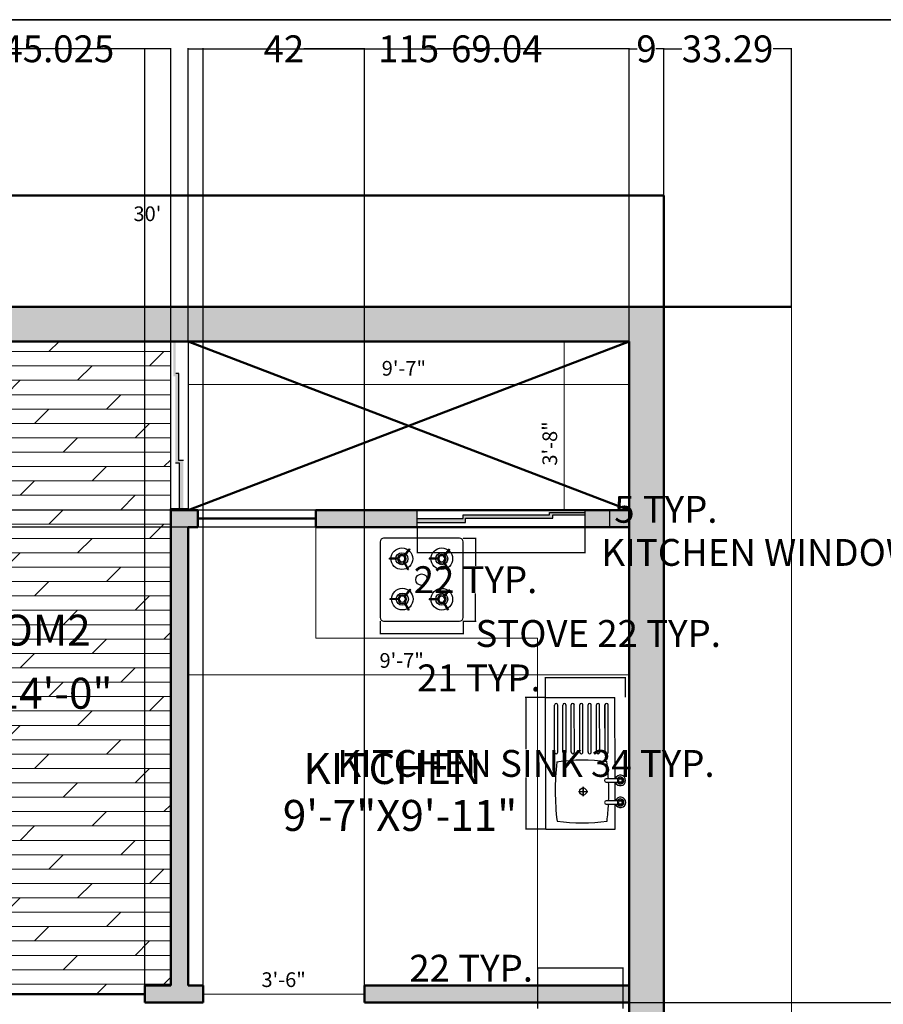
# Model space of a CAD drawing. Units: inches. Extents: x 1381 to 2246, y 1317 to 2168.
# Tile 8 of 15: x 1579 to 1804, y 1911 to 2168. Entities that reach past the tile are written whole.
import ezdxf

# ---------------------------------------------------------------- set-up
doc = ezdxf.new("R2010")
doc.units = ezdxf.units.IN
doc.header["$MEASUREMENT"] = 0
doc.layers.get('0').update_dxf_attribs({"color": 253})
for name, color, linetype, lineweight in [('A-ANNO-DIMS', 2, 'Continuous', 18), ('A-ANNO-TEXT', 7, 'Continuous', 18), ('A-ANNO-TTLB', 7, 'Continuous', 35), ('A-AREA-IDEN', 3, 'Continuous', 25), ('A-FLOR-FIXT', 9, 'Continuous', 18), ('A-FLOR-PATT', 252, 'Continuous', 13), ('A-FURN', 8, 'Continuous', 18), ('A-GLAZ', 4, 'Continuous', 25), ('A-WALL', 7, 'Continuous', 50)]:
    doc.layers.add(name, color=color, linetype=linetype, lineweight=lineweight)
doc.layers.add('furniture', color=250, linetype='Continuous')
doc.styles.get("Standard").update_dxf_attribs({"font": 'arial.ttf'})
doc.dimstyles.get("Standard").update_dxf_attribs({"dimtxt": 7, "dimasz": 0.18, "dimexe": 0.18, "dimexo": 0.0625, "dimgap": 0.09, "dimtad": 0, "dimtih": 1, "dimtoh": 1, "dimdec": 1, "dimzin": 0, "dimdsep": 46, "dimlunit": 3, "dimtxsty": 'Standard', "dimcen": 0.09, "dimadec": 0, "dimazin": 0, "dimtfac": 1, "dimtdec": 1, "dimtofl": 0, "dimtmove": 0, "dimatfit": 3, "dimfxl": 1, "dimtolj": 1, "dimtzin": 0, "dimarcsym": 0})

# ---------------------------------------------------------------- blocks, each defined once
blk = doc.blocks.new('4bstove')
at = {"layer": 'furniture'}
for p, q in [((1452.73, 1446.21), (1452.73, 1448.61)), ((1452.98, 1446.22), (1452.98, 1448.61)), ((1464.44, 1446.34), (1464.44, 1448.73)), ((1464.69, 1446.34), (1464.69, 1448.73)), ((1451.74, 1444.45), (1449.67, 1443.25)), ((1451.87, 1444.23), (1449.79, 1443.04)), ((1453.75, 1444.08), (1455.58, 1442.54)), ((1453.91, 1444.27), (1455.74, 1442.73)), ((1463.45, 1444.58), (1461.38, 1443.38)), ((1463.57, 1444.36), (1461.5, 1443.17)), ((1465.46, 1444.21), (1467.29, 1442.67)), ((1465.62, 1444.4), (1467.45, 1442.86)), ((1452.69, 1434.81), (1452.69, 1437.2)), ((1452.94, 1434.81), (1452.94, 1437.2)), ((1464.44, 1434.81), (1464.44, 1437.2)), ((1464.69, 1434.81), (1464.69, 1437.2)), ((1451.7, 1433.04), (1449.63, 1431.85)), ((1451.82, 1432.83), (1449.75, 1431.63)), ((1453.71, 1432.67), (1455.54, 1431.13)), ((1453.87, 1432.86), (1455.7, 1431.33)), ((1463.45, 1433.04), (1461.38, 1431.85)), ((1463.57, 1432.83), (1461.5, 1431.63)), ((1465.46, 1432.67), (1467.29, 1431.13)), ((1465.62, 1432.86), (1467.45, 1431.33))]:
    blk.add_line(p, q, dxfattribs=at)
for points in [[(1447.5, 1427.38), (1469.5, 1427.38, 0.414214), (1470.5, 1428.38), (1470.5, 1450.38, 0.414214), (1469.5, 1451.38), (1447.5, 1451.38, 0.414214), (1446.5, 1450.38), (1446.5, 1428.38, 0.414214)], [(1453.75, 1444.97, 1), (1452, 1444.97, 1)], [(1465.46, 1445.1, 1), (1463.71, 1445.1, 1)], [(1453.71, 1433.56, 1), (1451.96, 1433.56, 1)], [(1465.46, 1433.56, 1), (1463.71, 1433.56, 1)]]:
    blk.add_lwpolyline(points, format="xyb", close=True, dxfattribs=at)
for points in [[(1454.12, 1444.97, 1), (1451.62, 1444.97, 1), (1454.12, 1444.97, 1)], [(1465.83, 1445.1, 1), (1463.33, 1445.1, 1), (1465.83, 1445.1, 1)], [(1454.08, 1433.56, 1), (1451.58, 1433.56, 1), (1454.08, 1433.56, 1)], [(1465.83, 1433.56, 1), (1463.33, 1433.56, 1), (1465.83, 1433.56, 1)]]:
    blk.add_lwpolyline(points, format="xyb", dxfattribs=at)
for centre, radius in [((1452.87, 1444.97), 3.14), ((1464.58, 1445.1), 3.14), ((1452.87, 1444.97), 1.75), ((1464.58, 1445.1), 1.75), ((1458.5, 1439.38), 1.67), ((1452.83, 1433.56), 3.14), ((1464.58, 1433.56), 3.14), ((1452.83, 1433.56), 1.75), ((1464.58, 1433.56), 1.75)]:
    blk.add_circle(centre, radius, dxfattribs=at)
for centre, start, end in [((1452.87, 1444.97), 88.2645, 92.2039), ((1464.58, 1445.1), 88.2645, 92.2039), ((1452.87, 1444.97), 208.188, 212.1274), ((1452.87, 1444.97), 318.1018, 322.0412), ((1464.58, 1445.1), 208.188, 212.1274), ((1464.58, 1445.1), 318.1018, 322.0412), ((1452.83, 1433.56), 88.2645, 92.2039), ((1464.58, 1433.56), 88.2645, 92.2039)]:
    blk.add_arc(centre, 3.64, start, end, dxfattribs=at)
blk = doc.blocks.new('stove')
at = {"layer": 'furniture', "xscale": 0.9, "yscale": 0.9, "zscale": 0.9, "rotation": 89.99999999999999}
blk.add_blockref('4bstove', (1295.44, -1312.65), dxfattribs=at)
blk = doc.blocks.new('A$C799204C7')
for p, q in [((0, 34.2), (17.99, 34.2)), ((0, 0), (0, 34.2)), ((17.99, 13.08), (17.99, 34.2)), ((2.32, 20.01), (2.32, 32.27)), ((3.13, 20.01), (3.13, 32.27)), ((4.48, 20.01), (4.48, 32.27)), ((5.29, 20.01), (5.29, 32.27)), ((6.64, 20.01), (6.64, 32.27)), ((7.45, 20.01), (7.45, 32.27)), ((8.85, 20.01), (8.85, 32.27)), ((9.66, 20.01), (9.66, 32.27)), ((11.01, 20.01), (11.01, 32.27)), ((11.82, 20.01), (11.82, 32.27)), ((13.22, 20.01), (13.22, 32.27)), ((14.03, 20.01), (14.03, 32.27)), ((15.42, 20.01), (15.42, 32.27)), ((16.24, 20.01), (16.24, 32.27)), ((18.59, 13.08), (15.71, 13.08)), ((9.73, 11), (9.73, 8.54)), ((15.71, 12.17), (18.59, 12.17)), ((17.99, 7.36), (17.99, 12.17)), ((8.52, 9.77), (10.9, 9.77)), ((18.59, 7.36), (15.71, 7.36)), ((15.71, 6.45), (18.59, 6.45)), ((17.99, 0), (17.99, 6.45)), ((0, 0), (17.99, 0))]:
    blk.add_line(p, q)
for centre, radius in [((19.38, 12.62), 0.684), ((19.38, 12.62), 0.456), ((9.7, 9.77), 0.916), ((19.38, 6.91), 0.684), ((19.38, 6.91), 0.456)]:
    blk.add_circle(centre, radius)
for centre, radius, start, end in [((2.72, 32.27), 0.407, 0, 180), ((4.88, 32.27), 0.407, 0, 180), ((7.05, 32.27), 0.407, 0, 180), ((9.25, 32.27), 0.407, 0, 180), ((11.42, 32.27), 0.407, 0, 180), ((13.62, 32.27), 0.407, 0, 180), ((15.83, 32.27), 0.407, 0, 180), ((2.72, 20.01), 0.407, 180, 0), ((4.88, 20.01), 0.407, 180, 0), ((7.05, 20.01), 0.407, 180, 0), ((9.25, 20.01), 0.407, 180, 0), ((11.42, 20.01), 0.407, 180, 0), ((13.62, 20.01), 0.407, 180, 0), ((15.83, 20.01), 0.407, 180, 0), ((67.33, 9.77), 64.88, 173.1952, 186.8048), ((9.53, -30.19), 48.1, 82.3437, 97.8966), ((-48.51, 9.77), 64.88, 2.9208, 6.8048), ((15.71, 12.62), 0.456, 90, 270), ((19.38, 12.62), 1.37, 199.6514, 160.3603), ((19.38, 12.62), 0.911, 210.3431, 149.7554), ((-48.51, 9.77), 64.88, 357.8723, 2.115), ((19.38, 6.91), 1.37, 199.6514, 160.3603), ((19.38, 6.91), 0.911, 210.3431, 149.7554), ((15.71, 6.91), 0.456, 90, 270), ((-48.51, 9.77), 64.88, 353.1952, 357.0665), ((9.53, 49.73), 48.1, 262.1034, 277.6563)]:
    blk.add_arc(centre, radius, start, end)
blk = doc.blocks.new('sink')
at = {"layer": 'furniture'}
for p, q in [((8718164203.894819, -1433730582.369047), (8718164201.504578, -1433730582.369047)), ((8718164202.684322, -1433730581.131674), (8718164202.684322, -1433730583.598095)), ((8718164196.150837, -1433730592.638258), (8718164196.150837, -1433730604.938997)), ((8718164196.967728, -1433730592.638258), (8718164196.967728, -1433730604.938997)), ((8718164198.365185, -1433730592.638258), (8718164198.365185, -1433730604.938997)), ((8718164199.182076, -1433730592.638258), (8718164199.182076, -1433730604.938997)), ((8718164200.579533, -1433730592.638258), (8718164200.579533, -1433730604.938997)), ((8718164201.396423, -1433730592.638258), (8718164201.396423, -1433730604.938997)), ((8718164202.748692, -1433730592.638258), (8718164202.748692, -1433730604.938997)), ((8718164203.565582, -1433730592.638258), (8718164203.565582, -1433730604.938997)), ((8718164204.963041, -1433730592.638258), (8718164204.963041, -1433730604.938997)), ((8718164205.779934, -1433730592.638258), (8718164205.779934, -1433730604.938997)), ((8718164207.1322, -1433730592.638258), (8718164207.1322, -1433730604.938997)), ((8718164207.949093, -1433730592.638258), (8718164207.949093, -1433730604.938997)), ((8718164209.301359, -1433730592.638258), (8718164209.301359, -1433730604.938997)), ((8718164210.118252, -1433730592.638258), (8718164210.118252, -1433730604.938997))]:
    blk.add_line(p, q, dxfattribs=at)
for centre, radius in [((8718164192.998869, -1433730579.495552), 0.685789), ((8718164192.998869, -1433730579.495552), 0.457192), ((8718164202.715019, -1433730582.369047), 0.919003), ((8718164192.998869, -1433730585.228166), 0.68579), ((8718164192.998869, -1433730585.228166), 0.68579), ((8718164192.998869, -1433730585.228166), 0.457192)]:
    blk.add_circle(centre, radius, dxfattribs=at)
for centre, radius, start, end in [((8718164196.559284, -1433730592.638258), 0.41045, 354.3355999, 185.6644001), ((8718164198.77363, -1433730592.638258), 0.41045, 354.3355999, 185.6644001), ((8718164200.98798, -1433730592.638258), 0.41045, 354.3355999, 185.6644001), ((8718164203.157139, -1433730592.638258), 0.41045, 354.3355999, 185.6644001), ((8718164205.371487, -1433730592.638258), 0.41045, 354.3355999, 185.6644001), ((8718164207.540646, -1433730592.640262), 0.41045, 354.3355999, 185.6644001), ((8718164209.709805, -1433730592.640262), 0.41045, 354.3355999, 185.6644001), ((8718164196.559284, -1433730604.938997), 0.408445, 180, 0), ((8718164198.77363, -1433730604.938997), 0.408445, 180, 0), ((8718164200.98798, -1433730604.938997), 0.408445, 180, 0), ((8718164203.157139, -1433730604.938997), 0.408445, 180, 0), ((8718164205.371487, -1433730604.938997), 0.408445, 180, 0), ((8718164207.540646, -1433730604.938997), 0.408445, 180, 0), ((8718164209.709805, -1433730604.938997), 0.408445, 180, 0)]:
    blk.add_arc(centre, radius, start, end, dxfattribs=at)
at = {"layer": 'furniture', "xscale": 1.0032, "yscale": 1.0032, "zscale": 1.0032, "rotation": 180}
blk.add_blockref('A$C799204C7', (8718164212.441259, -1433730572.566334), dxfattribs=at)
blk = doc.blocks.new('washbasin')
at = {"layer": 'furniture'}
blk.add_blockref('sink', (-8718164214.119328, 1433730589.721069), dxfattribs=at)
blk = doc.blocks.new('WIN-KITCHEN')
for p, q in [((0, 0), (0, 4.5)), ((0, 4.5), (43.68, 4.5)), ((43.68, 4.5), (43.68, 0)), ((43.68, 0), (0, 0))]:
    blk.add_line(p, q)
blk = doc.blocks.new('*D30')
at = {"layer": 'A-ANNO-DIMS', "color": 0, "lineweight": -2, "transparency": 16777216}
for p, q in [((1713.7, 1920.4), (1713.52, 1920.4)), ((1713.7, 1909.87), (1713.7, 1920.58)), ((1735.75, 1920.4), (1713.88, 1920.4)), ((1735.93, 1909.87), (1735.93, 1920.58))]:
    blk.add_line(p, q, dxfattribs=at)
at = {"layer": 'A-ANNO-DIMS', "color": 0, "transparency": 16777216}
for points in [[(1713.88, 1920.43), (1713.88, 1920.37), (1713.7, 1920.4)], [(1735.75, 1920.43), (1735.75, 1920.37), (1735.93, 1920.4)]]:
    blk.add_solid(points, dxfattribs=at)
at = {"layer": 'Defpoints', "color": 0, "transparency": 16777216}
for p in [(1713.7, 1920.4), (1713.7, 1909.81), (1735.93, 1909.81)]:
    blk.add_point(p, dxfattribs=at)
at = {"layer": 'A-ANNO-DIMS', "color": 0, "transparency": 16777216, "insert": (1696.34, 1920.4), "char_height": 7, "attachment_point": 5}
blk.add_mtext('\\A1;22 TYP.', dxfattribs=at)
blk = doc.blocks.new('*D31')
at = {"layer": 'A-ANNO-DIMS', "color": 0, "lineweight": -2, "transparency": 16777216}
for p, q in [((1672.63, 2010.89), (1672.63, 2007.53)), ((1694.23, 2010.89), (1694.23, 2007.53)), ((1672.81, 2007.71), (1694.05, 2007.71)), ((1694.23, 2007.71), (1694.41, 2007.71))]:
    blk.add_line(p, q, dxfattribs=at)
at = {"layer": 'A-ANNO-DIMS', "color": 0, "transparency": 16777216}
for points in [[(1672.81, 2007.74), (1672.81, 2007.68), (1672.63, 2007.71)], [(1694.05, 2007.74), (1694.05, 2007.68), (1694.23, 2007.71)]]:
    blk.add_solid(points, dxfattribs=at)
at = {"layer": 'Defpoints', "color": 0, "transparency": 16777216}
for p in [(1672.63, 2010.95), (1694.23, 2010.95), (1694.23, 2007.71)]:
    blk.add_point(p, dxfattribs=at)
at = {"layer": 'A-ANNO-DIMS', "color": 0, "transparency": 16777216, "insert": (1729.46, 2007.71), "char_height": 7, "attachment_point": 5}
blk.add_mtext('\\A1;STOVE 22 TYP.', dxfattribs=at)
blk = doc.blocks.new('*D32')
at = {"layer": 'A-ANNO-DIMS', "color": 0, "lineweight": -2, "transparency": 16777216}
for p, q in [((1694.3, 2032.55), (1697.65, 2032.55)), ((1697.47, 2032.37), (1697.47, 2025.36)), ((1697.47, 2011.13), (1697.47, 2018.14)), ((1694.3, 2010.95), (1697.65, 2010.95))]:
    blk.add_line(p, q, dxfattribs=at)
at = {"layer": 'A-ANNO-DIMS', "color": 0, "transparency": 16777216}
for points in [[(1697.44, 2032.37), (1697.5, 2032.37), (1697.47, 2032.55)], [(1697.44, 2011.13), (1697.5, 2011.13), (1697.47, 2010.95)]]:
    blk.add_solid(points, dxfattribs=at)
at = {"layer": 'Defpoints', "color": 0, "transparency": 16777216}
for p in [(1694.23, 2032.55), (1697.47, 2032.55), (1694.23, 2010.95)]:
    blk.add_point(p, dxfattribs=at)
at = {"layer": 'A-ANNO-DIMS', "color": 0, "transparency": 16777216, "insert": (1697.47, 2021.75), "char_height": 7, "attachment_point": 5}
blk.add_mtext('\\A1;22 TYP.', dxfattribs=at)
blk = doc.blocks.new('*D33')
at = {"layer": 'A-ANNO-DIMS', "color": 0, "lineweight": -2, "transparency": 16777216}
for p, q in [((1715.69, 1990.99), (1710.43, 1990.98)), ((1710.61, 1990.8), (1710.63, 1977.53)), ((1710.67, 1956.85), (1710.65, 1970.11)), ((1715.75, 1956.68), (1710.49, 1956.67))]:
    blk.add_line(p, q, dxfattribs=at)
at = {"layer": 'A-ANNO-DIMS', "color": 0, "transparency": 16777216}
for points in [[(1710.64, 1990.8), (1710.58, 1990.8), (1710.61, 1990.98)], [(1710.7, 1956.85), (1710.64, 1956.85), (1710.67, 1956.67)]]:
    blk.add_solid(points, dxfattribs=at)
at = {"layer": 'Defpoints', "color": 0, "transparency": 16777216}
for p in [(1715.75, 1990.99), (1710.67, 1956.67), (1715.82, 1956.68)]:
    blk.add_point(p, dxfattribs=at)
at = {"layer": 'A-ANNO-DIMS', "color": 0, "transparency": 16777216, "insert": (1710.64, 1973.82), "char_height": 7, "attachment_point": 5}
blk.add_mtext('\\A1;KITCHEN SINK 34 TYP.', dxfattribs=at)
blk = doc.blocks.new('*D34')
at = {"layer": 'A-ANNO-DIMS', "color": 0, "lineweight": -2, "transparency": 16777216}
for p, q in [((1715.75, 1996.13), (1715.57, 1996.13)), ((1715.75, 1991.05), (1715.75, 1996.31)), ((1736.38, 1996.17), (1715.93, 1996.13)), ((1736.57, 1991.09), (1736.56, 1996.35))]:
    blk.add_line(p, q, dxfattribs=at)
at = {"layer": 'A-ANNO-DIMS', "color": 0, "transparency": 16777216}
for points in [[(1715.93, 1996.16), (1715.93, 1996.1), (1715.75, 1996.13)], [(1736.38, 1996.2), (1736.38, 1996.14), (1736.56, 1996.17)]]:
    blk.add_solid(points, dxfattribs=at)
at = {"layer": 'Defpoints', "color": 0, "transparency": 16777216}
for p in [(1715.75, 1996.13), (1715.75, 1990.99), (1736.57, 1991.02)]:
    blk.add_point(p, dxfattribs=at)
at = {"layer": 'A-ANNO-DIMS', "color": 0, "transparency": 16777216, "insert": (1698.38, 1996.13), "char_height": 7, "attachment_point": 5}
blk.add_mtext('\\A1;21 TYP.', dxfattribs=at)
blk = doc.blocks.new('*D37')
at = {"layer": 'A-ANNO-DIMS', "color": 0, "lineweight": -2, "transparency": 16777216}
for p, q in [((1690.35, 1893.74), (1690.35, 1890.53)), ((1710.95, 1893.74), (1710.95, 1890.53)), ((1690.53, 1890.71), (1710.77, 1890.71)), ((1710.95, 1890.71), (1711.13, 1890.71))]:
    blk.add_line(p, q, dxfattribs=at)
at = {"layer": 'A-ANNO-DIMS', "color": 0, "transparency": 16777216}
for points in [[(1690.53, 1890.74), (1690.53, 1890.68), (1690.35, 1890.71)], [(1710.77, 1890.74), (1710.77, 1890.68), (1710.95, 1890.71)]]:
    blk.add_solid(points, dxfattribs=at)
at = {"layer": 'Defpoints', "color": 0, "transparency": 16777216}
for p in [(1690.35, 1893.8), (1710.95, 1893.8), (1710.95, 1890.71)]:
    blk.add_point(p, dxfattribs=at)
at = {"layer": 'A-ANNO-DIMS', "color": 0, "transparency": 16777216, "insert": (1748.72, 1890.71), "char_height": 7, "attachment_point": 5}
blk.add_mtext('\\A1;TV UNIT 21 TYP.', dxfattribs=at)
blk = doc.blocks.new('*D41')
at = {"layer": 'A-ANNO-DIMS', "color": 0, "lineweight": -2, "transparency": 16777216}
for p, q in [((1682.28, 2035.35), (1682.28, 2028.68)), ((1725.96, 2035.35), (1725.96, 2028.68)), ((1682.46, 2028.86), (1725.78, 2028.86)), ((1725.96, 2028.86), (1726.14, 2028.86))]:
    blk.add_line(p, q, dxfattribs=at)
at = {"layer": 'A-ANNO-DIMS', "color": 0, "transparency": 16777216}
for points in [[(1682.46, 2028.89), (1682.46, 2028.83), (1682.28, 2028.86)], [(1725.78, 2028.89), (1725.78, 2028.83), (1725.96, 2028.86)]]:
    blk.add_solid(points, dxfattribs=at)
at = {"layer": 'Defpoints', "color": 0, "transparency": 16777216}
for p in [(1682.28, 2035.42), (1725.96, 2035.42), (1725.96, 2028.86)]:
    blk.add_point(p, dxfattribs=at)
at = {"layer": 'A-ANNO-DIMS', "color": 0, "transparency": 16777216, "insert": (1788.75, 2028.86), "char_height": 7, "attachment_point": 5}
blk.add_mtext('\\A1;KITCHEN WINDOW 44 TYP.', dxfattribs=at)
blk = doc.blocks.new('*D42')
at = {"layer": 'A-ANNO-DIMS', "color": 0, "lineweight": -2, "transparency": 16777216}
for p, q in [((1726.03, 2039.92), (1732.7, 2039.92)), ((1732.52, 2039.92), (1732.52, 2040.1)), ((1732.52, 2040.1), (1732.7, 2040.1)), ((1732.52, 2035.6), (1732.52, 2039.74)), ((1726.03, 2035.42), (1732.7, 2035.42))]:
    blk.add_line(p, q, dxfattribs=at)
at = {"layer": 'A-ANNO-DIMS', "color": 0, "transparency": 16777216}
for points in [[(1732.49, 2039.74), (1732.55, 2039.74), (1732.52, 2039.92)], [(1732.49, 2035.6), (1732.55, 2035.6), (1732.52, 2035.42)]]:
    blk.add_solid(points, dxfattribs=at)
at = {"layer": 'Defpoints', "color": 0, "transparency": 16777216}
for p in [(1725.96, 2039.92), (1732.52, 2039.92), (1725.96, 2035.42)]:
    blk.add_point(p, dxfattribs=at)
at = {"layer": 'A-ANNO-DIMS', "color": 0, "transparency": 16777216, "insert": (1747.1, 2040.1), "char_height": 7, "attachment_point": 5}
blk.add_mtext('\\A1;5 TYP.', dxfattribs=at)
blk = doc.blocks.new('*D52')
at = {"layer": 'A-ANNO-DIMS', "color": 0, "lineweight": -2, "transparency": 16777216}
for p, q in [((1746.55, 2092.98), (1746.55, 2160.41)), ((1746.73, 2160.23), (1751.29, 2160.23)), ((1779.66, 2160.23), (1775.1, 2160.23)), ((1779.84, 2092.98), (1779.84, 2160.41))]:
    blk.add_line(p, q, dxfattribs=at)
at = {"layer": 'A-ANNO-DIMS', "color": 0, "transparency": 16777216}
for points in [[(1746.73, 2160.26), (1746.73, 2160.2), (1746.55, 2160.23)], [(1779.66, 2160.26), (1779.66, 2160.2), (1779.84, 2160.23)]]:
    blk.add_solid(points, dxfattribs=at)
at = {"layer": 'Defpoints', "color": 0, "transparency": 16777216}
for p in [(1779.84, 2160.23), (1746.55, 2092.92), (1779.84, 2092.92)]:
    blk.add_point(p, dxfattribs=at)
at = {"layer": 'A-ANNO-DIMS', "color": 0, "transparency": 16777216, "insert": (1763.2, 2160.23), "char_height": 7, "attachment_point": 5}
blk.add_mtext('\\A1;33.29', dxfattribs=at)
blk = doc.blocks.new('*D58')
at = {"layer": 'A-ANNO-DIMS', "color": 0, "lineweight": -2, "transparency": 16777216}
for p, q in [((1456.05, 2083.98), (1456.05, 2160.41)), ((1456.23, 2160.23), (1529.59, 2160.23)), ((1617.87, 2160.23), (1544.51, 2160.23)), ((1618.05, 2083.98), (1618.05, 2160.41))]:
    blk.add_line(p, q, dxfattribs=at)
at = {"layer": 'A-ANNO-DIMS', "color": 0, "transparency": 16777216}
for points in [[(1456.23, 2160.26), (1456.23, 2160.2), (1456.05, 2160.23)], [(1617.87, 2160.26), (1617.87, 2160.2), (1618.05, 2160.23)]]:
    blk.add_solid(points, dxfattribs=at)
at = {"layer": 'Defpoints', "color": 0, "transparency": 16777216}
for p in [(1618.05, 2160.23), (1456.05, 2083.92), (1618.05, 2083.92)]:
    blk.add_point(p, dxfattribs=at)
at = {"layer": 'A-ANNO-DIMS', "color": 0, "transparency": 16777216, "insert": (1537.05, 2160.23), "char_height": 7, "attachment_point": 5}
blk.add_mtext('\\A1;162', dxfattribs=at)
blk = doc.blocks.new('*D59')
at = {"layer": 'A-ANNO-DIMS', "color": 0, "lineweight": -2, "transparency": 16777216}
for p, q in [((1622.55, 2083.98), (1622.55, 2160.41)), ((1622.73, 2160.23), (1672.53, 2160.23)), ((1737.37, 2160.23), (1687.57, 2160.23)), ((1737.55, 2083.98), (1737.55, 2160.41))]:
    blk.add_line(p, q, dxfattribs=at)
at = {"layer": 'A-ANNO-DIMS', "color": 0, "transparency": 16777216}
for points in [[(1622.73, 2160.26), (1622.73, 2160.2), (1622.55, 2160.23)], [(1737.37, 2160.26), (1737.37, 2160.2), (1737.55, 2160.23)]]:
    blk.add_solid(points, dxfattribs=at)
at = {"layer": 'Defpoints', "color": 0, "transparency": 16777216}
for p in [(1737.55, 2160.23), (1622.55, 2083.92), (1737.55, 2083.92)]:
    blk.add_point(p, dxfattribs=at)
at = {"layer": 'A-ANNO-DIMS', "color": 0, "transparency": 16777216, "insert": (1680.05, 2160.23), "char_height": 7, "attachment_point": 5}
blk.add_mtext('\\A1;115', dxfattribs=at)
blk = doc.blocks.new('*D61')
at = {"layer": 'A-ANNO-DIMS', "color": 0, "lineweight": -2, "transparency": 16777216}
for p, q in [((1737.61, 1911.42), (1818.27, 1911.42)), ((1818.09, 1911.24), (1818.09, 1808.63)), ((1818.09, 1698.7), (1818.09, 1801.3)), ((1737.61, 1698.52), (1818.27, 1698.52))]:
    blk.add_line(p, q, dxfattribs=at)
at = {"layer": 'A-ANNO-DIMS', "color": 0, "transparency": 16777216}
for points in [[(1818.06, 1911.24), (1818.12, 1911.24), (1818.09, 1911.42)], [(1818.06, 1698.7), (1818.12, 1698.7), (1818.09, 1698.52)]]:
    blk.add_solid(points, dxfattribs=at)
at = {"layer": 'Defpoints', "color": 0, "transparency": 16777216}
for p in [(1737.55, 1911.42), (1818.09, 1911.42), (1737.55, 1698.52)]:
    blk.add_point(p, dxfattribs=at)
at = {"layer": 'A-ANNO-DIMS', "color": 0, "transparency": 16777216, "insert": (1818.09, 1804.97), "char_height": 7, "attachment_point": 5}
blk.add_mtext('\\A1;212.9', dxfattribs=at)
blk = doc.blocks.new('*D69')
at = {"layer": 'A-ANNO-DIMS', "color": 0, "lineweight": -2, "transparency": 16777216}
for p, q in [((1737.55, 2083.98), (1737.55, 2160.41)), ((1737.73, 2160.23), (1739.66, 2160.23)), ((1746.37, 2160.23), (1744.44, 2160.23)), ((1746.55, 2092.98), (1746.55, 2160.41))]:
    blk.add_line(p, q, dxfattribs=at)
at = {"layer": 'A-ANNO-DIMS', "color": 0, "transparency": 16777216}
for points in [[(1737.73, 2160.26), (1737.73, 2160.2), (1737.55, 2160.23)], [(1746.37, 2160.26), (1746.37, 2160.2), (1746.55, 2160.23)]]:
    blk.add_solid(points, dxfattribs=at)
at = {"layer": 'Defpoints', "color": 0, "transparency": 16777216}
for p in [(1746.55, 2160.23), (1746.55, 2092.92), (1737.55, 2083.92)]:
    blk.add_point(p, dxfattribs=at)
at = {"layer": 'A-ANNO-DIMS', "color": 0, "transparency": 16777216, "insert": (1742.05, 2160.23), "char_height": 7, "attachment_point": 5}
blk.add_mtext('\\A1;9', dxfattribs=at)
blk = doc.blocks.new('*D70')
at = {"layer": 'A-ANNO-DIMS', "color": 0, "lineweight": -2, "transparency": 16777216}
for p, q in [((1655.76, 2039.92), (1408.62, 2039.92)), ((1408.8, 2039.74), (1408.8, 2035.6)), ((1655.76, 2035.42), (1408.62, 2035.42)), ((1408.8, 2035.24), (1408.62, 2035.24)), ((1408.8, 2035.42), (1408.8, 2035.24))]:
    blk.add_line(p, q, dxfattribs=at)
at = {"layer": 'A-ANNO-DIMS', "color": 0, "transparency": 16777216}
for points in [[(1408.77, 2039.74), (1408.83, 2039.74), (1408.8, 2039.92)], [(1408.77, 2035.6), (1408.83, 2035.6), (1408.8, 2035.42)]]:
    blk.add_solid(points, dxfattribs=at)
at = {"layer": 'Defpoints', "color": 0, "transparency": 16777216}
for p in [(1655.82, 2039.92), (1408.8, 2035.42), (1655.82, 2035.42)]:
    blk.add_point(p, dxfattribs=at)
at = {"layer": 'A-ANNO-DIMS', "color": 0, "transparency": 16777216, "insert": (1401.99, 2035.24), "char_height": 7, "attachment_point": 5}
blk.add_mtext('\\A1;4.5', dxfattribs=at)
blk = doc.blocks.new('*D72')
at = {"layer": 'A-ANNO-DIMS', "color": 0, "lineweight": -2, "transparency": 16777216}
for p, q in [((1566.21, 1911.48), (1566.21, 2160.41)), ((1566.39, 2160.23), (1573.94, 2160.23)), ((1611.06, 2160.23), (1603.51, 2160.23)), ((1611.24, 1911.48), (1611.24, 2160.41))]:
    blk.add_line(p, q, dxfattribs=at)
at = {"layer": 'A-ANNO-DIMS', "color": 0, "transparency": 16777216}
for points in [[(1566.39, 2160.26), (1566.39, 2160.2), (1566.21, 2160.23)], [(1611.06, 2160.26), (1611.06, 2160.2), (1611.24, 2160.23)]]:
    blk.add_solid(points, dxfattribs=at)
at = {"layer": 'Defpoints', "color": 0, "transparency": 16777216}
for p in [(1611.24, 2160.23), (1566.21, 1911.42), (1611.24, 1911.42)]:
    blk.add_point(p, dxfattribs=at)
at = {"layer": 'A-ANNO-DIMS', "color": 0, "transparency": 16777216, "insert": (1588.72, 2160.23), "char_height": 7, "attachment_point": 5}
blk.add_mtext('\\A1;45.025', dxfattribs=at)
blk = doc.blocks.new('*D73')
at = {"layer": 'A-ANNO-DIMS', "color": 0, "lineweight": -2, "transparency": 16777216}
for p, q in [((1626.51, 1911.48), (1626.51, 2160.41)), ((1626.69, 2160.23), (1642.3, 2160.23)), ((1668.33, 2160.23), (1652.72, 2160.23)), ((1668.51, 1911.48), (1668.51, 2160.41))]:
    blk.add_line(p, q, dxfattribs=at)
at = {"layer": 'A-ANNO-DIMS', "color": 0, "transparency": 16777216}
for points in [[(1626.69, 2160.26), (1626.69, 2160.2), (1626.51, 2160.23)], [(1668.33, 2160.26), (1668.33, 2160.2), (1668.51, 2160.23)]]:
    blk.add_solid(points, dxfattribs=at)
at = {"layer": 'Defpoints', "color": 0, "transparency": 16777216}
for p in [(1668.51, 2160.23), (1626.51, 1911.42), (1668.51, 1911.42)]:
    blk.add_point(p, dxfattribs=at)
at = {"layer": 'A-ANNO-DIMS', "color": 0, "transparency": 16777216, "insert": (1647.51, 2160.23), "char_height": 7, "attachment_point": 5}
blk.add_mtext('\\A1;42', dxfattribs=at)
blk = doc.blocks.new('*D74')
at = {"layer": 'A-ANNO-DIMS', "color": 0, "lineweight": -2, "transparency": 16777216}
for p, q in [((1668.51, 1911.48), (1668.51, 2160.41)), ((1668.69, 2160.23), (1691.13, 2160.23)), ((1737.37, 2160.23), (1714.94, 2160.23)), ((1737.55, 1911.48), (1737.55, 2160.41))]:
    blk.add_line(p, q, dxfattribs=at)
at = {"layer": 'A-ANNO-DIMS', "color": 0, "transparency": 16777216}
for points in [[(1668.69, 2160.26), (1668.69, 2160.2), (1668.51, 2160.23)], [(1737.37, 2160.26), (1737.37, 2160.2), (1737.55, 2160.23)]]:
    blk.add_solid(points, dxfattribs=at)
at = {"layer": 'Defpoints', "color": 0, "transparency": 16777216}
for p in [(1737.55, 2160.23), (1668.51, 1911.42), (1737.55, 1911.42)]:
    blk.add_point(p, dxfattribs=at)
at = {"layer": 'A-ANNO-DIMS', "color": 0, "transparency": 16777216, "insert": (1703.03, 2160.23), "char_height": 7, "attachment_point": 5}
blk.add_mtext('\\A1;69.04', dxfattribs=at)

msp = doc.modelspace()

# ---------------------------------------------------------------- hatches: boundary and pattern name
at = {"layer": 'A-FLOR-PATT'}
h = msp.add_hatch(dxfattribs=at)
h.set_pattern_fill('DOLMIT', color=256, scale=15)
h.paths.add_polyline_path([(1618.051, 2040.2358), (1618.051, 2083.9163), (1517.1194, 2083.9163), (1517.1194, 2057.4148), (1456.051, 2057.4148), (1456.051, 1915.9163), (1478.9621, 1915.9163), (1478.9621, 1913.6663), (1511.016, 1913.6663), (1511.016, 1915.9163), (1566.2107, 1915.9163), (1566.2107, 1913.6663), (1611.2353, 1913.6663), (1611.2353, 1915.9163), (1618.051, 1915.9163)])
h.paths.add_polyline_path([(1526.2629, 2024.4608), (1526.2629, 1955.9789), (1497.7075, 1955.9789), (1497.7075, 1962.7697), (1471.5798, 1962.7697), (1471.6908, 1951.263), (1458.495, 1951.263), (1458.384, 1962.7697), (1458.384, 2014.1291), (1458.273, 2025.6358), (1471.4689, 2025.6358), (1471.5798, 2014.1291), (1497.7075, 2014.1291), (1497.7075, 2024.4608)], flags=16)
h.paths.add_polyline_path([(1475.9437, 2014.0737), (1475.9437, 2004.8072), (1469.1114, 2004.8072), (1469.0654, 2004.7449), (1469.0654, 1968.5691), (1461.3046, 1968.5691), (1461.3046, 1983.6181), (1469.0654, 1983.6181), (1469.0654, 1989.7582), (1461.3046, 1989.7582), (1461.3046, 2004.8072), (1469.1114, 2004.8072)], flags=0)
h.paths.add_polyline_path([(1469.1187, 2020.1923, -1), (1460.6232, 2020.1923, -1)], flags=0)
h.paths.add_polyline_path([(1469.2296, 1957.3262, -1), (1460.7342, 1957.3262, -1)], flags=0)
h.paths.add_polyline_path([(1533.5744, 1985.8776), (1602.6925, 1985.8776), (1602.6925, 1998.2538), (1533.5744, 1998.2538)], flags=24)
h.paths.add_polyline_path([(1535.349, 2002.3157), (1604.0842, 2002.3157), (1604.0842, 2014.8488), (1535.349, 2014.8488)], flags=24)
at = {"layer": 'A-GLAZ'}
h = msp.add_hatch(color=256, dxfattribs=at)
h.dxf.hatch_style = 1
h.paths.add_polyline_path([(1456.051, 2083.9163), (1737.551, 2083.9163), (1737.551, 1677.4163), (1732.8596, 1677.4163), (1732.8596, 1672.9163), (1737.551, 1672.9163), (1737.551, 1471.9163), (1746.551, 1471.9163), (1746.551, 2092.9163), (1447.051, 2092.9163), (1447.051, 2083.9163), (1447.051, 1471.9163), (1488.6632, 1471.9163), (1488.6632, 1480.9163), (1456.051, 1480.9163), (1456.051, 1710.4163), (1517.1194, 1710.4163), (1517.1194, 1714.9163), (1491.551, 1714.9163), (1491.551, 1729.193), (1487.051, 1729.193), (1487.051, 1714.9163), (1456.051, 1714.9163)])
h.paths.add_polyline_path([(1622.551, 2035.4163), (1625.0954, 2035.4163), (1625.0954, 2039.9163), (1618.051, 2039.9163), (1618.051, 1915.9163), (1611.2353, 1915.9163), (1611.2353, 1911.4163), (1626.5102, 1911.4163), (1626.5102, 1915.9163), (1622.551, 1915.9163)], flags=17)
h.paths.add_polyline_path([(1737.551, 1915.9163), (1668.5102, 1915.9163), (1668.5102, 1911.4163), (1737.551, 1911.4163)], flags=17)
h.paths.add_polyline_path([(1682.2831, 2039.9163), (1655.8191, 2039.9163), (1655.8191, 2035.4163), (1682.2831, 2035.4163)], flags=17)
h.paths.add_polyline_path([(1737.551, 2039.9163), (1725.9636, 2039.9163), (1725.9636, 2035.4163), (1737.551, 2035.4163)], flags=17)
h.paths.add_polyline_path([(1684.2508, 1711.4667), (1740.8192, 1711.4667), (1740.8192, 1723.8346), (1684.2508, 1723.8346)], flags=25)
h = msp.add_hatch(color=256, dxfattribs=at)
h.dxf.hatch_style = 1
h.paths.add_polyline_path([(1620.1648, 2052.8139), (1620.1648, 2075.5544), (1619.3285, 2075.5544), (1619.3285, 2083.9163), (1618.6665, 2083.9163), (1618.6665, 2074.7522), (1619.2588, 2074.7522), (1619.2588, 2052.1861), (1620.301, 2052.1861), (1620.301, 2040.2358), (1621.3147, 2040.2358), (1621.3147, 2052.8139)])
h = msp.add_hatch(color=256, dxfattribs=at)
h.dxf.hatch_style = 1
h.paths.add_polyline_path([(1694.8612, 2037.8025), (1717.6017, 2037.8025), (1717.6017, 2038.6388), (1725.9636, 2038.6388), (1725.9636, 2039.3008), (1716.7995, 2039.3008), (1716.7995, 2038.7085), (1694.2334, 2038.7085), (1694.2334, 2037.6663), (1682.2831, 2037.6663), (1682.2831, 2036.6526), (1694.8612, 2036.6526)])

# ---------------------------------------------------------------- linework, layer by layer
at = {"layer": 'A-ANNO-DIMS'}
for p, q in [((1779.8404, 2092.9163), (1779.8404, 1471.9163)), ((1720.6176, 2083.9163), (1720.6176, 2039.9163)), ((1622.551, 2072.6853), (1737.551, 2072.6853)), ((1622.551, 1996.9422), (1737.551, 1996.9422)), ((1626.5102, 1913.6663), (1668.5102, 1913.6663))]:
    msp.add_line(p, q, dxfattribs=at)
at = {"layer": 'A-ANNO-TTLB'}
msp.add_line((1380.9518, 2167.8236), (2244.072, 2167.8236), dxfattribs=at)
at = {"layer": 'A-FURN'}
for p, q in [((1655.8191, 2035.4163), (1655.8191, 2006.4935)), ((1655.8191, 2006.4935), (1713.5964, 2006.4935)), ((1713.5964, 2006.4935), (1713.5964, 1915.9163))]:
    msp.add_line(p, q, dxfattribs=at)
at = {"layer": 'A-GLAZ'}
for p, q in [((1618.051, 2083.9163), (1622.551, 2083.9163)), ((1618.051, 2039.9163), (1618.051, 2083.9163)), ((1618.051, 2083.9163), (1622.551, 2083.9163)), ((1618.051, 2083.9163), (1622.551, 2083.9163)), ((1622.551, 2083.9163), (1622.551, 2040.2358)), ((1620.1648, 2075.5544), (1619.3285, 2075.5544)), ((1620.1648, 2052.8139), (1620.1648, 2075.5544)), ((1620.301, 2052.1861), (1619.2588, 2052.1861)), ((1621.3147, 2052.8139), (1620.1648, 2052.8139)), ((1620.301, 2040.2358), (1620.301, 2052.1861)), ((1622.551, 2040.2358), (1618.051, 2040.2358)), ((1716.7995, 2038.7085), (1716.7995, 2039.3008)), ((1716.7995, 2039.3008), (1725.9636, 2039.3008)), ((1682.2831, 2037.6663), (1694.2334, 2037.6663)), ((1694.2334, 2037.6663), (1694.2334, 2038.7085)), ((1694.2334, 2038.7085), (1716.7995, 2038.7085)), ((1694.8612, 2036.6526), (1694.8612, 2037.8025)), ((1694.8612, 2037.8025), (1717.6017, 2037.8025)), ((1717.6017, 2037.8025), (1717.6017, 2038.6388)), ((1717.6017, 2038.6388), (1725.9636, 2038.6388)), ((1682.2831, 2036.6526), (1694.8612, 2036.6526)), ((1668.5102, 1913.6663), (1668.5102, 1913.6663))]:
    msp.add_line(p, q, dxfattribs=at)
at = {"layer": 'A-WALL'}
for p, q in [((1447.051, 2121.9832), (1746.551, 2121.9832)), ((1746.551, 2121.9832), (1746.551, 2092.9163)), ((1779.8404, 2092.9163), (1447.051, 2092.9163)), ((1456.051, 2092.9163), (1746.551, 2092.9163)), ((1746.551, 2092.9163), (1746.551, 1471.9163)), ((1746.551, 2092.9163), (1779.8404, 2092.9163)), ((1779.8404, 2092.9163), (1746.551, 2092.9163)), ((1456.051, 2083.9163), (1737.551, 2083.9163)), ((1622.551, 2083.9163), (1737.551, 2039.9163)), ((1622.551, 2039.9163), (1737.551, 2083.9163)), ((1737.551, 2083.9163), (1737.551, 1677.4163)), ((1618.051, 2040.2358), (1618.051, 1915.9163)), ((1618.051, 2039.9163), (1625.0954, 2039.9163)), ((1622.551, 2040.2358), (1622.551, 2039.9163)), ((1625.0954, 2039.9163), (1625.0954, 2035.4163)), ((1655.8191, 2039.9163), (1655.8191, 2035.4163)), ((1655.8191, 2039.9163), (1737.551, 2039.9163)), ((1625.0954, 2037.6663), (1655.8191, 2037.6663)), ((1622.551, 2035.4163), (1625.0954, 2035.4163)), ((1622.551, 2035.4163), (1622.551, 1915.9163)), ((1655.8191, 2035.4163), (1737.551, 2035.4163)), ((1566.2107, 1913.6663), (1611.2353, 1913.6663)), ((1611.2353, 1915.9163), (1611.2353, 1911.4163)), ((1611.2353, 1915.9163), (1618.051, 1915.9163)), ((1622.551, 1915.9163), (1626.5102, 1915.9163)), ((1626.5102, 1915.9163), (1626.5102, 1911.4163)), ((1668.5102, 1913.6663), (1668.5102, 1915.9163)), ((1668.5102, 1915.9163), (1668.5102, 1911.4163)), ((1668.5102, 1915.9163), (1737.551, 1915.9163)), ((1611.2353, 1911.4163), (1611.2353, 1911.4163)), ((1611.2353, 1911.4163), (1626.5102, 1911.4163)), ((1668.5102, 1911.4163), (1737.551, 1911.4163))]:
    msp.add_line(p, q, dxfattribs=at)

# ---------------------------------------------------------------- block references
at = {"layer": 'A-FLOR-FIXT'}
msp.add_blockref('stove', (1683.4334, 2021.7494), dxfattribs=at)
at = {"layer": 'A-FLOR-FIXT', "rotation": 180.1045348756012}
msp.add_blockref('washbasin', (1714.1082, 1973.8279), dxfattribs=at)
at = {"layer": 'A-GLAZ'}
msp.add_blockref('WIN-KITCHEN', (1682.283, 2035.416), dxfattribs=at)

# ---------------------------------------------------------------- texts
at = {"layer": 'A-ANNO-TEXT'}
for s, p in [("30'", (1608.3132, 2115.2823)), ('9\'-7"', (1673.0232, 2074.9732)), ('9\'-7"', (1672.4524, 1998.7616)), ('3\'-6"', (1641.6797, 1915.4983))]:
    msp.add_text(s, height=3.83139, dxfattribs=at).set_placement(p)
msp.add_text('3\'-8"', height=3.83139, rotation=90, dxfattribs=at).set_placement((1718.7517, 2051.5078))
at = {"layer": 'A-AREA-IDEN'}
for s, height, p in [('BEDROOM2', 8.07451, (1537.4378, 2004.5422)), ('13\'-6"X14\'-0"', 8.074511, (1535.6371, 1988.0835)), ('KITCHEN', 8.07451, (1652.6455, 1968.4525)), ('9\'-7"X9\'-11"', 8.074511, (1647.2515, 1956.2128))]:
    msp.add_text(s, height=height, dxfattribs=at).set_placement(p)

# ---------------------------------------------------------------- dimensions: what is measured, and where the dimension line sits
at = {"layer": 'A-ANNO-DIMS'}
for base, p1, p2, override, picture, middle in [((1618.051, 2160.2332), (1456.051, 2083.9163), (1618.051, 2083.9163), {"dimdec": 0, "dimlfac": 1, "dimrnd": 0, "dimzin": 0, "dimdsep": 46, "dimlunit": 2}, '*D58', (1537.051, 2160.2332)), ((1611.2353, 2160.2332), (1566.2107, 1911.4163), (1611.2353, 1911.4163), {"dimdec": 3, "dimlfac": 1, "dimrnd": 0, "dimzin": 0, "dimdsep": 46, "dimlunit": 2}, '*D72', (1588.723, 2160.2332)), ((1737.551, 2160.2332), (1622.551, 2083.9163), (1737.551, 2083.9163), {"dimdec": 0, "dimlfac": 1, "dimrnd": 0, "dimzin": 0, "dimdsep": 46, "dimlunit": 2}, '*D59', (1680.051, 2160.2332)), ((1668.5102, 2160.2332), (1626.5102, 1911.4163), (1668.5102, 1911.4163), {"dimdec": 0, "dimlfac": 1, "dimrnd": 0, "dimzin": 0, "dimdsep": 46, "dimlunit": 2}, '*D73', (1647.5102, 2160.2332)), ((1737.551, 2160.2332), (1668.5102, 1911.4163), (1737.551, 1911.4163), {"dimdec": 2, "dimlfac": 1, "dimrnd": 0, "dimzin": 0, "dimdsep": 46, "dimlunit": 2}, '*D74', (1703.0306, 2160.2332)), ((1746.551, 2160.2332), (1737.551, 2083.9163), (1746.551, 2092.9163), {"dimdec": 0, "dimlfac": 1, "dimrnd": 0, "dimzin": 0, "dimdsep": 46, "dimlunit": 2}, '*D69', (1742.051, 2160.2332)), ((1779.8404, 2160.2332), (1746.551, 2092.9163), (1779.8404, 2092.9163), {"dimdec": 2, "dimlfac": 1, "dimrnd": 0, "dimzin": 0, "dimdsep": 46, "dimlunit": 2}, '*D52', (1763.1957, 2160.2332))]:
    dim = msp.add_linear_dim(base=base, p1=p1, p2=p2, dimstyle='Standard', override=override, dxfattribs=at)
    dim.commit()
    dim.dimension.update_dxf_attribs({"geometry": picture, "text_midpoint": middle})
for base, p1, p2, text, picture, middle in [((1725.9636, 2028.8642), (1682.2831, 2035.4163), (1725.9636, 2035.4163), 'KITCHEN WINDOW <> TYP.', '*D41', (1788.7466, 2028.8642)), ((1694.2334, 2007.7094), (1672.6334, 2010.9494), (1694.2334, 2010.9494), 'STOVE <> TYP.', '*D31', (1729.4556, 2007.7094)), ((1710.9534, 1890.7089), (1690.3532, 1893.799), (1710.9534, 1893.799), 'TV UNIT <> TYP.', '*D37', (1748.7207, 1890.7089))]:
    dim = msp.add_linear_dim(base=base, p1=p1, p2=p2, text=text, dimstyle='Standard', override={"dimdec": 0, "dimrnd": 0, "dimzin": 0, "dimlunit": 2}, dxfattribs=at)
    dim.commit()
    dim.dimension.update_dxf_attribs({"geometry": picture, "text_midpoint": middle})
for base, p1, p2, angle, text, picture, middle in [((1732.5156685922, 2039.9163125031), (1725.9635957099, 2035.4163125031), (1725.9635957099, 2039.9163125031), 90, '<> TYP.', '*D42', (1747.103199288, 2040.0963125031)), ((1697.4734, 2032.5494), (1694.2334, 2010.9494), (1694.2334, 2032.5494), 90, '<> TYP.', '*D32', (1697.4734, 2021.7494)), ((1715.7456, 1996.132), (1736.569, 1991.0236), (1715.755, 1990.9856), 180.104535, '<> TYP.', '*D34', (1698.3791, 1996.1317)), ((1710.6712, 1956.6669), (1715.755, 1990.9856), (1715.8176, 1956.6763), 270.104535, 'KITCHEN SINK <> TYP.', '*D33', (1710.6399, 1973.8216)), ((1713.702, 1920.4021), (1735.931, 1909.8106), (1713.702, 1909.8106), 180, '<> TYP.', '*D30', (1696.3354, 1920.4021))]:
    dim = msp.add_linear_dim(base=base, p1=p1, p2=p2, angle=angle, text=text, dimstyle='Standard', override={"dimdec": 0, "dimrnd": 0, "dimzin": 0, "dimlunit": 2}, dxfattribs=at)
    dim.commit()
    dim.dimension.update_dxf_attribs({"geometry": picture, "text_midpoint": middle})
for base, p1, p2, picture, middle in [((1408.801, 2035.4163), (1655.8191, 2039.9163), (1655.8191, 2035.4163), '*D70', (1401.9918, 2035.2363)), ((1818.0904, 1911.4163), (1737.551, 1698.5169), (1737.551, 1911.4163), '*D61', (1818.0904, 1804.9666))]:
    dim = msp.add_linear_dim(base=base, p1=p1, p2=p2, angle=90, dimstyle='Standard', override={"dimdec": 1, "dimlfac": 1, "dimrnd": 0, "dimzin": 0, "dimdsep": 46, "dimlunit": 2}, dxfattribs=at)
    dim.commit()
    dim.dimension.update_dxf_attribs({"geometry": picture, "text_midpoint": middle})

doc.saveas('drawing.dxf')
